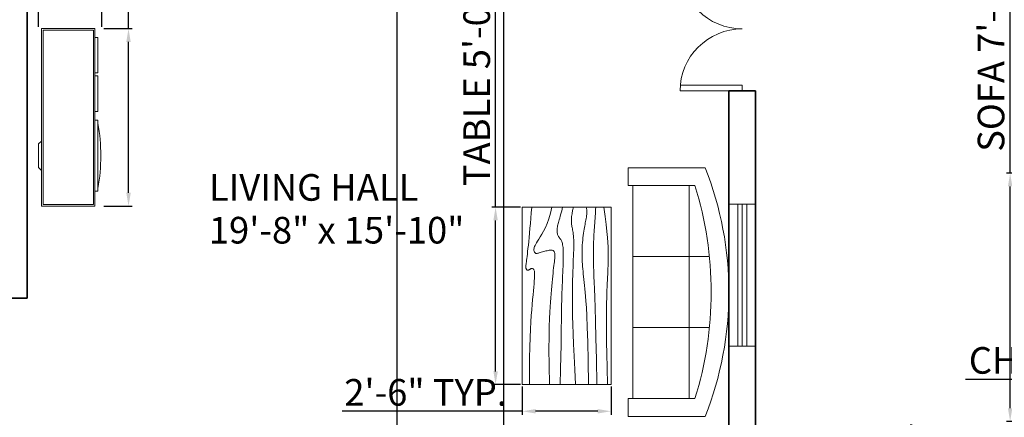
# Model space of a CAD drawing. Units: inches. Extents: x 2081 to 4786, y 1256 to 3802.
# Tile 4 of 7: x 2352 to 2685, y 1670 to 1804. Entities that reach past the tile are written whole.
import ezdxf

# ---------------------------------------------------------------- set-up
doc = ezdxf.new("R2010")
doc.units = ezdxf.units.IN
for name, color, linetype, lineweight in [('A-ANNO-DIMS', 18, 'Continuous', 18), ('A-AREA-IDEN', 18, 'Continuous', 18), ('A-DOOR', 5, 'Continuous', 18), ('A-FURN', 5, 'Continuous', 18), ('A-GLAZ', 11, 'Continuous', 18), ('A-WALL', 7, 'Continuous', 35)]:
    doc.layers.add(name, color=color, linetype=linetype, lineweight=lineweight)
doc.styles.get("Standard").update_dxf_attribs({"font": 'arial.ttf'})
doc.dimstyles.new('ISO-25', dxfattribs={"dimtxt": 9, "dimasz": 4.5, "dimexe": 1.25, "dimexo": 0.625, "dimtad": 1, "dimdec": 0, "dimlunit": 3, "dimtxsty": 'Standard', "dimcen": 2.5, "dimadec": 0, "dimazin": 0, "dimtfac": 1, "dimtdec": 0, "dimtmove": 0, "dimatfit": 3, "dimfxl": 1, "dimarcsym": 0})

# ---------------------------------------------------------------- blocks, each defined once
blk = doc.blocks.new('Sofa - Roundback 7 ft.')
for p, q in [((-12.00002, -32.4421), (-12.00003, -6.5971)), ((11.99997, -32.4421), (11.99998, -6.5971)), ((-36.000027, -34), (-36.000027, -11.4696)), ((35.99998, -34), (35.99998, -11.4696)), ((-35.999844, -13.3819), (35.9998, -13.3819)), ((-36.000027, -32.4421), (35.99998, -32.4421))]:
    blk.add_line(p, q)
for points in [[(-36.000027, -34), (-42.000027, -34), (-42.000027, -8)], [(41.99998, -8), (41.99998, -34), (35.99998, -34)]]:
    blk.add_lwpolyline(points)
for centre, radius, start, end in [((0, -114.25), 114.25, 68.43141, 111.5686), ((-0.00001, -127.1968), 121.1968, 72.72033, 107.2797)]:
    blk.add_arc(centre, radius, start, end)
blk = doc.blocks.new('Table - Rectangular Woodgrain 60 x 30 in.')
for p, q in [((0, 0), (0, -30)), ((60, 0), (0, 0)), ((60, -30), (60, 0)), ((0, -30), (60, -30))]:
    blk.add_line(p, q)
for points in [[(0, -2.4), (4.8155, -2.418), (9.0302, -2.4688), (12.709, -2.5477), (15.9167, -2.65), (18.7181, -2.7711), (21.1781, -2.9063), (23.3616, -3.0508), (25.3333, -3.2), (27.1477, -3.3495), (28.8172, -3.4958), (30.3437, -3.636), (31.7291, -3.7667), (32.9756, -3.8849), (34.0849, -3.9875), (35.059, -4.0714), (35.9, -4.1334), (36.6114, -4.1711), (37.2041, -4.1854), (37.6906, -4.1779), (38.0833, -4.15), (38.3948, -4.1034), (38.6375, -4.0396), (38.8239, -3.9602), (38.9666, -3.8667), (39.0764, -3.7608), (39.1573, -3.6448), (39.2116, -3.521), (39.2416, -3.3917), (39.2498, -3.2593), (39.2385, -3.1261), (39.21, -2.9944), (39.1666, -2.8667), (39.111, -2.7447), (39.0468, -2.6281), (38.978, -2.5163), (38.9083, -2.4083), (38.8418, -2.3035), (38.7823, -2.201), (38.7337, -2.1001), (38.7, -2), (38.6844, -1.9003), (38.6875, -1.8021), (38.7094, -1.707), (38.75, -1.6167), (38.8094, -1.5326), (38.8875, -1.4563), (38.9844, -1.3893), (39.1, -1.3333), (39.2351, -1.2896), (39.3937, -1.2583), (39.5804, -1.2396), (39.8, -1.2333), (40.057, -1.2396), (40.3562, -1.2583), (40.7023, -1.2896), (41.1, -1.3333), (41.5547, -1.3895), (42.0755, -1.4573), (42.6721, -1.5361), (43.3542, -1.625), (44.1316, -1.7233), (45.014, -1.8302), (46.0114, -1.9449), (47.1333, -2.0667), (48.3862, -2.1947), (49.7625, -2.3281), (51.2513, -2.4663), (52.8416, -2.6083), (54.5226, -2.7535), (56.2833, -2.9011), (58.1127, -3.0501), (60, -3.2)], [(0, -9.2), (6.5759, -9.0858), (11.9385, -9.0365), (16.2527, -9.0418), (19.6833, -9.0917), (22.3952, -9.1759), (24.5531, -9.2844), (26.322, -9.4069), (27.8666, -9.5333), (29.3241, -9.6553), (30.7203, -9.7719), (32.0532, -9.8837), (33.3208, -9.9917), (34.5213, -10.0965), (35.6526, -10.199), (36.7128, -10.2999), (37.7, -10.4), (38.6129, -10.4996), (39.4531, -10.5969), (40.223, -10.6895), (40.925, -10.775), (41.5613, -10.8512), (42.1344, -10.9156), (42.6465, -10.966), (43.1, -11), (43.4976, -11.0158), (43.8437, -11.0136), (44.143, -10.9942), (44.4, -10.9583), (44.6195, -10.9069), (44.8062, -10.8406), (44.9648, -10.7603), (45.1, -10.6667), (45.2155, -10.5598), (45.3114, -10.4365), (45.3871, -10.2929), (45.4416, -10.125), (45.4743, -9.929), (45.4844, -9.7011), (45.4709, -9.4371), (45.4333, -9.1333), (45.3716, -8.7883), (45.2896, -8.4104), (45.1919, -8.0107), (45.0833, -7.6), (44.9685, -7.1893), (44.8521, -6.7896), (44.7388, -6.4117), (44.6333, -6.0667), (44.54, -5.7628), (44.4614, -5.4979), (44.4001, -5.2675), (44.3583, -5.0667), (44.3384, -4.8909), (44.3427, -4.7354), (44.3736, -4.5956), (44.4333, -4.4667), (44.5236, -4.3453), (44.6427, -4.2333), (44.7884, -4.1339), (44.9583, -4.05), (45.1501, -3.9849), (45.3614, -3.9417), (45.59, -3.9234), (45.8333, -3.9333), (46.0915, -3.9749), (46.3734, -4.0531), (46.6906, -4.1736), (47.0542, -4.3417), (47.4756, -4.5629), (47.9661, -4.8427), (48.5372, -5.1866), (49.2, -5.6), (49.9676, -6.0844), (50.8594, -6.625), (51.8965, -7.2031), (53.1, -7.8), (54.491, -8.3969), (56.0906, -8.975), (57.9199, -9.5156), (60, -10)], [(0, -12.8), (5.1847, -12.9322), (9.6213, -13.0323), (13.3963, -13.1059), (16.5958, -13.1583), (19.3063, -13.1952), (21.614, -13.2219), (23.6054, -13.2439), (25.3666, -13.2667), (26.9728, -13.2947), (28.4531, -13.3281), (29.8256, -13.3663), (31.1083, -13.4083), (32.3191, -13.4535), (33.476, -13.501), (34.597, -13.5501), (35.7, -13.6), (36.7984, -13.6497), (37.8875, -13.6979), (38.9578, -13.743), (40, -13.7833), (41.0047, -13.8174), (41.9625, -13.8438), (42.864, -13.8607), (43.7, -13.8667), (44.4631, -13.8604), (45.1552, -13.8417), (45.7801, -13.8104), (46.3416, -13.7667), (46.8439, -13.7104), (47.2906, -13.6417), (47.6858, -13.5604), (48.0333, -13.4667), (48.3375, -13.3608), (48.6042, -13.2448), (48.8396, -13.121), (49.05, -12.9917), (49.2417, -12.8593), (49.4208, -12.7261), (49.5937, -12.5944), (49.7667, -12.4667), (49.9452, -12.3451), (50.1323, -12.2313), (50.3303, -12.1268), (50.5416, -12.0333), (50.7686, -11.9524), (51.0135, -11.8854), (51.2788, -11.8341), (51.5666, -11.8), (51.8785, -11.7843), (52.2116, -11.7865), (52.562, -11.8059), (52.926, -11.8417), (53.2998, -11.8931), (53.6795, -11.9594), (54.0614, -12.0397), (54.4416, -12.1333), (54.8223, -12.2401), (55.2293, -12.3625), (55.6942, -12.5037), (56.2489, -12.6667), (56.9251, -12.8547), (57.7545, -13.0708), (58.7689, -13.3182), (60, -13.6)], [(0, -18), (5.124, -17.7273), (9.6609, -17.5057), (13.6705, -17.3303), (17.2125, -17.1958), (20.3467, -17.0973), (23.1328, -17.0297), (25.6307, -16.9878), (27.9, -16.9667), (29.9928, -16.9617), (31.9302, -16.9703), (33.7254, -16.9907), (35.3917, -17.0208), (36.9423, -17.0588), (38.3906, -17.1026), (39.7499, -17.1503), (41.0333, -17.2), (42.2519, -17.2496), (43.4073, -17.2969), (44.4986, -17.3395), (45.525, -17.375), (46.4858, -17.4012), (47.3802, -17.4156), (48.2074, -17.416), (48.9667, -17.4), (49.6583, -17.3662), (50.2872, -17.3167), (50.8595, -17.2547), (51.3812, -17.1833), (51.8584, -17.1057), (52.2971, -17.025), (52.7034, -16.9443), (53.0833, -16.8667), (53.443, -16.7951), (53.789, -16.7313), (54.128, -16.6768), (54.4666, -16.6334), (54.8115, -16.6024), (55.1693, -16.5854), (55.5465, -16.5841), (55.95, -16.6), (56.3828, -16.6337), (56.8346, -16.6823), (57.2915, -16.7418), (57.7396, -16.8084), (58.165, -16.878), (58.5539, -16.9469), (58.8924, -17.0111), (59.1666, -17.0667), (59.3679, -17.1107), (59.5078, -17.1438), (59.6032, -17.1675), (59.6708, -17.1833), (59.7275, -17.193), (59.7901, -17.1979), (59.8753, -17.1998), (60, -17.2)], [(0, -22.4), (8.0098, -22.2501), (14.4094, -22.1011), (19.4168, -21.9535), (23.25, -21.8083), (26.1269, -21.6663), (28.2656, -21.5281), (29.884, -21.3947), (31.2, -21.2667), (32.3967, -21.1448), (33.5172, -21.0292), (34.5697, -20.9198), (35.5625, -20.8167), (36.5037, -20.7198), (37.4015, -20.6292), (38.2642, -20.5448), (39.1, -20.4667), (39.9164, -20.3951), (40.7187, -20.3313), (41.5117, -20.2768), (42.3, -20.2333), (43.0883, -20.2024), (43.8812, -20.1854), (44.6836, -20.1841), (45.5, -20.2), (46.3328, -20.234), (47.1747, -20.2844), (48.0163, -20.3488), (48.8479, -20.425), (49.66, -20.5106), (50.4429, -20.6031), (51.1872, -20.7004), (51.8833, -20.8), (52.5246, -20.8999), (53.1166, -20.9995), (53.6681, -21.0983), (54.1875, -21.1958), (54.6834, -21.2919), (55.1646, -21.3859), (55.6394, -21.4777), (56.1167, -21.5667), (56.6028, -21.6515), (57.0961, -21.7266), (57.5929, -21.7852), (58.0896, -21.8208), (58.5823, -21.8268), (59.0674, -21.7964), (59.5412, -21.723), (60, -21.6)], [(0, -25.2), (8.6355, -25.0504), (15.7026, -24.9031), (21.4049, -24.7606), (25.9458, -24.625), (29.529, -24.4988), (32.3578, -24.3844), (34.6359, -24.284), (36.5667, -24.2), (38.3213, -24.1341), (39.9417, -24.0854), (41.437, -24.0523), (42.8167, -24.0333), (44.0901, -24.0268), (45.2667, -24.0313), (46.3557, -24.0451), (47.3667, -24.0667), (48.309, -24.0947), (49.1928, -24.1287), (50.0284, -24.168), (50.826, -24.2125), (51.5959, -24.2617), (52.3483, -24.3151), (53.0935, -24.3725), (53.8417, -24.4334), (54.6009, -24.497), (55.3699, -24.561), (56.1454, -24.6226), (56.9239, -24.6792), (57.7021, -24.7279), (58.4764, -24.7662), (59.2435, -24.7911), (60, -24.8)], [(0, -28.8), (5.6867, -28.6681), (10.45, -28.5698), (14.407, -28.5012), (17.675, -28.4584), (20.3711, -28.4374), (22.6125, -28.4344), (24.5164, -28.4455), (26.2, -28.4667), (27.762, -28.4947), (29.2276, -28.5281), (30.6033, -28.5663), (31.8958, -28.6084), (33.1118, -28.6535), (34.2578, -28.7011), (35.3405, -28.7501), (36.3666, -28.8), (37.3443, -28.8497), (38.288, -28.8974), (39.2137, -28.9412), (40.1375, -28.9792), (41.0753, -29.0093), (42.0432, -29.0297), (43.0572, -29.0384), (44.1333, -29.0333), (45.2936, -29.0114), (46.5843, -28.9641), (48.0579, -28.8816), (49.7666, -28.7542), (51.7629, -28.5721), (54.0989, -28.3255), (56.8272, -28.0048), (60, -27.6)]]:
    blk.add_lwpolyline(points)
blk = doc.blocks.new('Entertainment Center')
for p, q in [((-4, 0), (-5, -1)), ((4, 0), (-4, 0)), ((5, -1), (4, 0)), ((-17, -19), (-17, -1)), ((-17, -1), (43, -1)), ((-16.5, -18.5), (-16.5, -1.5)), ((-16.5, -1.5), (42.5, -1.5)), ((42.5, -1.5), (42.5, -18.5)), ((43, -1), (43, -19)), ((43, -19), (-17, -19)), ((42.5, -18.5), (-16.5, -18.5)), ((-12, -20), (-12, -19)), ((12, -19), (12, -20)), ((15, -20), (15, -19)), ((27, -19), (27, -20)), ((28, -20), (28, -19)), ((40, -19), (40, -20)), ((12, -20), (-12, -20)), ((27, -20), (15, -20)), ((40, -20), (28, -20))]:
    blk.add_line(p, q)
blk.add_arc((0, 40), 61, 259.6111, 280.3889)
blk = doc.blocks.new('DOOR-PAIR-42IN')
for p, q in [((0, 42), (21, 42)), ((0, 40), (21, 40)), ((21, 42), (21, 40)), ((0, 2), (21, 2)), ((21, 0), (21, 2)), ((0, 0), (21, 0))]:
    blk.add_line(p, q)
for centre, start, end in [((21, 42), 180, 270), ((21, 0), 90, 180)]:
    blk.add_arc(centre, 21, start, end)
blk = doc.blocks.new('WINDOW-48IN')
for p, q in [((0, 0), (0, 9)), ((0, 9), (4, 9)), ((4, 9), (48, 9)), ((48, 0), (48, 9)), ((48, 6), (0, 6)), ((48, 4.5), (0, 4.5)), ((48, 3), (0, 3)), ((48, 0), (0, 0))]:
    blk.add_line(p, q)
blk = doc.blocks.new('*D51')
at = {"layer": 'A-ANNO-DIMS', "color": 0, "lineweight": -2, "transparency": 16777216}
for p, q in [((2744.09, 1682.64), (2671.91, 1682.64)), ((2744.09, 1677.68), (2744.09, 1683.89)), ((2776.84, 1682.64), (2748.59, 1682.64)), ((2781.34, 1677.68), (2781.34, 1683.89))]:
    blk.add_line(p, q, dxfattribs=at)
at = {"layer": 'A-ANNO-DIMS', "color": 0, "transparency": 16777216}
for points in [[(2748.59, 1683.39), (2748.59, 1681.89), (2744.09, 1682.64)], [(2776.84, 1683.39), (2776.84, 1681.89), (2781.34, 1682.64)]]:
    blk.add_solid(points, dxfattribs=at)
at = {"layer": 'Defpoints', "color": 0, "transparency": 16777216}
for p in [(2744.09, 1682.64), (2744.09, 1677.06), (2781.34, 1677.06)]:
    blk.add_point(p, dxfattribs=at)
at = {"layer": 'A-ANNO-DIMS', "color": 0, "transparency": 16777216, "insert": (2705.75, 1687.93), "char_height": 9, "attachment_point": 5}
blk.add_mtext('CHAIR 3\'-1"', dxfattribs=at)
blk = doc.blocks.new('*D55')
at = {"layer": 'A-ANNO-DIMS', "color": 0, "lineweight": -2, "transparency": 16777216}
for p, q in [((2686.95, 1752.41), (2686.95, 1850.7)), ((2698.93, 1752.41), (2685.7, 1752.41)), ((2686.95, 1672.91), (2686.95, 1747.91)), ((2698.93, 1668.41), (2685.7, 1668.41))]:
    blk.add_line(p, q, dxfattribs=at)
at = {"layer": 'A-ANNO-DIMS', "color": 0, "transparency": 16777216}
for points in [[(2686.2, 1747.91), (2687.7, 1747.91), (2686.95, 1752.41)], [(2686.2, 1672.91), (2687.7, 1672.91), (2686.95, 1668.41)]]:
    blk.add_solid(points, dxfattribs=at)
at = {"layer": 'Defpoints', "color": 0, "transparency": 16777216}
for p in [(2686.95, 1752.41), (2699.55, 1752.41), (2699.55, 1668.41)]:
    blk.add_point(p, dxfattribs=at)
at = {"layer": 'A-ANNO-DIMS', "color": 0, "transparency": 16777216, "insert": (2681.67, 1803.8), "char_height": 9, "attachment_point": 5, "rotation": 90}
blk.add_mtext('SOFA 7\'-0" TYP.', dxfattribs=at)
blk = doc.blocks.new('*D56')
at = {"layer": 'A-ANNO-DIMS', "color": 0, "lineweight": -2, "transparency": 16777216}
for p, q in [((2699.55, 1667.78), (2699.55, 1654.56)), ((2736.22, 1667.78), (2736.22, 1654.56)), ((2699.55, 1655.81), (2617.98, 1655.81)), ((2731.72, 1655.81), (2704.05, 1655.81))]:
    blk.add_line(p, q, dxfattribs=at)
at = {"layer": 'A-ANNO-DIMS', "color": 0, "transparency": 16777216}
for points in [[(2704.05, 1656.56), (2704.05, 1655.06), (2699.55, 1655.81)], [(2731.72, 1656.56), (2731.72, 1655.06), (2736.22, 1655.81)]]:
    blk.add_solid(points, dxfattribs=at)
at = {"layer": 'Defpoints', "color": 0, "transparency": 16777216}
for p in [(2699.55, 1668.41), (2736.22, 1668.41), (2699.55, 1655.81)]:
    blk.add_point(p, dxfattribs=at)
at = {"layer": 'A-ANNO-DIMS', "color": 0, "transparency": 16777216, "insert": (2656.52, 1661.09), "char_height": 9, "attachment_point": 5}
blk.add_mtext('3\'-0 1/2" TYP.', dxfattribs=at)
blk = doc.blocks.new('*D57')
at = {"layer": 'A-ANNO-DIMS', "color": 0, "lineweight": -2, "transparency": 16777216}
for p, q in [((2513.19, 1740.9), (2513.19, 1845.06)), ((2521.57, 1740.9), (2511.94, 1740.9)), ((2513.19, 1685.4), (2513.19, 1736.4)), ((2521.57, 1680.9), (2511.94, 1680.9))]:
    blk.add_line(p, q, dxfattribs=at)
at = {"layer": 'A-ANNO-DIMS', "color": 0, "transparency": 16777216}
for points in [[(2512.44, 1736.4), (2513.94, 1736.4), (2513.19, 1740.9)], [(2512.44, 1685.4), (2513.94, 1685.4), (2513.19, 1680.9)]]:
    blk.add_solid(points, dxfattribs=at)
at = {"layer": 'Defpoints', "color": 0, "transparency": 16777216}
for p in [(2513.19, 1740.9), (2522.19, 1740.9), (2522.19, 1680.9)]:
    blk.add_point(p, dxfattribs=at)
at = {"layer": 'A-ANNO-DIMS', "color": 0, "transparency": 16777216, "insert": (2507.97, 1795.23), "char_height": 9, "attachment_point": 5, "rotation": 90}
blk.add_mtext('TABLE 5\'-0" TYP.', dxfattribs=at)
blk = doc.blocks.new('*D58')
at = {"layer": 'A-ANNO-DIMS', "color": 0, "lineweight": -2, "transparency": 16777216}
for p, q in [((2522.19, 1680.27), (2522.19, 1670.65)), ((2552.19, 1680.27), (2552.19, 1670.65)), ((2522.19, 1671.9), (2461.43, 1671.9)), ((2547.69, 1671.9), (2526.69, 1671.9))]:
    blk.add_line(p, q, dxfattribs=at)
at = {"layer": 'A-ANNO-DIMS', "color": 0, "transparency": 16777216}
for points in [[(2526.69, 1672.65), (2526.69, 1671.15), (2522.19, 1671.9)], [(2547.69, 1672.65), (2547.69, 1671.15), (2552.19, 1671.9)]]:
    blk.add_solid(points, dxfattribs=at)
at = {"layer": 'Defpoints', "color": 0, "transparency": 16777216}
for p in [(2522.19, 1680.9), (2552.19, 1680.9), (2522.19, 1671.9)]:
    blk.add_point(p, dxfattribs=at)
at = {"layer": 'A-ANNO-DIMS', "color": 0, "transparency": 16777216, "insert": (2489.56, 1677.12), "char_height": 9, "attachment_point": 5}
blk.add_mtext('2\'-6" TYP.', dxfattribs=at)
blk = doc.blocks.new('*D59')
at = {"layer": 'A-ANNO-DIMS', "color": 0, "lineweight": -2, "transparency": 16777216}
for p, q in [((2389.23, 1801.25), (2389.23, 1937.59)), ((2380.85, 1801.25), (2390.48, 1801.25)), ((2389.23, 1745.75), (2389.23, 1796.75)), ((2380.85, 1741.25), (2390.48, 1741.25))]:
    blk.add_line(p, q, dxfattribs=at)
at = {"layer": 'A-ANNO-DIMS', "color": 0, "transparency": 16777216}
for points in [[(2388.48, 1796.75), (2389.98, 1796.75), (2389.23, 1801.25)], [(2388.48, 1745.75), (2389.98, 1745.75), (2389.23, 1741.25)]]:
    blk.add_solid(points, dxfattribs=at)
at = {"layer": 'Defpoints', "color": 0, "transparency": 16777216}
for p in [(2380.23, 1801.25), (2389.23, 1801.25), (2380.23, 1741.25)]:
    blk.add_point(p, dxfattribs=at)
at = {"layer": 'A-ANNO-DIMS', "color": 0, "transparency": 16777216, "insert": (2384.01, 1871.67), "char_height": 9, "attachment_point": 5, "rotation": 90}
blk.add_mtext('MEDIA UNIT 5\'-0" TYP.', dxfattribs=at)
blk = doc.blocks.new('*D60')
at = {"layer": 'A-ANNO-DIMS', "color": 0, "lineweight": -2, "transparency": 16777216}
for p, q in [((2358.89, 1810.25), (2278.16, 1810.25)), ((2358.89, 1801.88), (2358.89, 1811.5)), ((2375.73, 1810.25), (2363.39, 1810.25)), ((2380.23, 1801.88), (2380.23, 1811.5))]:
    blk.add_line(p, q, dxfattribs=at)
at = {"layer": 'A-ANNO-DIMS', "color": 0, "transparency": 16777216}
for points in [[(2363.39, 1811), (2363.39, 1809.5), (2358.89, 1810.25)], [(2375.73, 1811), (2375.73, 1809.5), (2380.23, 1810.25)]]:
    blk.add_solid(points, dxfattribs=at)
at = {"layer": 'Defpoints', "color": 0, "transparency": 16777216}
for p in [(2358.89, 1810.25), (2358.89, 1801.25), (2380.23, 1801.25)]:
    blk.add_point(p, dxfattribs=at)
at = {"layer": 'A-ANNO-DIMS', "color": 0, "transparency": 16777216, "insert": (2316.28, 1815.53), "char_height": 9, "attachment_point": 5}
blk.add_mtext('1\'-9 1/2" TYP.', dxfattribs=at)
blk = doc.blocks.new('*D78')
at = {"layer": 'A-ANNO-DIMS', "color": 0, "lineweight": -2, "transparency": 16777216}
for p, q in [((2479.98, 1626.8), (2479.98, 2072.92)), ((2484.48, 2071.67), (2511.48, 2071.67)), ((2515.98, 1639.8), (2515.98, 2072.92))]:
    blk.add_line(p, q, dxfattribs=at)
at = {"layer": 'A-ANNO-DIMS', "color": 0, "transparency": 16777216}
for points in [[(2484.48, 2072.42), (2484.48, 2070.92), (2479.98, 2071.67)], [(2511.48, 2072.42), (2511.48, 2070.92), (2515.98, 2071.67)]]:
    blk.add_solid(points, dxfattribs=at)
at = {"layer": 'Defpoints', "color": 0, "transparency": 16777216}
for p in [(2515.98, 2071.67), (2515.98, 1639.17), (2479.98, 1626.17)]:
    blk.add_point(p, dxfattribs=at)
at = {"layer": 'A-ANNO-DIMS', "color": 0, "transparency": 16777216, "insert": (2497.98, 2076.9), "char_height": 9, "attachment_point": 5}
blk.add_mtext('3\'-0"', dxfattribs=at)

msp = doc.modelspace()

# ---------------------------------------------------------------- linework, layer by layer
at = {"layer": 'A-WALL'}
for p, q in [((2354.98, 1710.17), (2354.98, 1834.17)), ((2591.98, 1780.17), (2600.98, 1780.17)), ((2591.98, 1644.17), (2591.98, 1780.17)), ((2600.98, 1433.17), (2600.98, 1780.17)), ((2343.98, 1710.17), (2354.98, 1710.17))]:
    msp.add_line(p, q, dxfattribs=at)

# ---------------------------------------------------------------- block references
at = {"layer": 'A-DOOR'}
msp.add_blockref('DOOR-PAIR-42IN', (2575.48, 1780.17), dxfattribs=at)
at = {"layer": 'A-FURN'}
for name, p, rotation in [('Entertainment Center', (2358.89, 1758.25), 90), ('Sofa - Roundback 7 ft.', (2591.98, 1712.17), 270), ('Table - Rectangular Woodgrain 60 x 30 in.', (2522.19, 1680.9), 90)]:
    msp.add_blockref(name, p, dxfattribs=dict(at, rotation=rotation))
at = {"layer": 'A-GLAZ', "rotation": 269.9999999999987}
msp.add_blockref('WINDOW-48IN', (2591.98, 1741.91), dxfattribs=at)

# ---------------------------------------------------------------- texts
at = {"layer": 'A-AREA-IDEN'}
for s, p in [('LIVING HALL', (2416.37, 1743.07)), ('19\'-8" x 15\'-10"', (2416.37, 1728.61))]:
    msp.add_text(s, height=9, dxfattribs=at).set_placement(p)

# ---------------------------------------------------------------- dimensions: what is measured, and where the dimension line sits
at = {"layer": 'A-ANNO-DIMS'}
dim = msp.add_linear_dim(base=(2515.98, 2071.67), p1=(2479.98, 1626.17), p2=(2515.98, 1639.17), dimstyle='ISO-25', override={"dimdec": 1, "dimlfac": 1, "dimrnd": 0, "dimzin": 1, "dimdsep": 46, "dimlunit": 4, "dimfrac": 2}, dxfattribs=at)
dim.commit()
dim.dimension.update_dxf_attribs({"geometry": '*D78', "text_midpoint": (2497.98, 2076.9)})
for base, p1, p2, angle, text, picture, middle in [((2389.23, 1801.25), (2380.23, 1741.25), (2380.23, 1801.25), 90, 'MEDIA UNIT <> TYP.', '*D59', (2384.01, 1871.67)), ((2686.95, 1752.41), (2699.55, 1668.41), (2699.55, 1752.41), 90, 'SOFA <> TYP.', '*D55', (2681.67, 1803.8)), ((2513.19, 1740.9), (2522.19, 1680.9), (2522.19, 1740.9), 90, 'TABLE <> TYP.', '*D57', (2507.97, 1795.23)), ((2358.89, 1810.25), (2380.23, 1801.25), (2358.89, 1801.25), 180, '<> TYP.', '*D60', (2316.28, 1815.53)), ((2744.0897, 1682.6449), (2781.3368, 1677.0579), (2744.0897, 1677.0579), 180, 'CHAIR <>', '*D51', (2705.7488, 1687.9265)), ((2522.19, 1671.9), (2552.19, 1680.9), (2522.19, 1680.9), 180, '<> TYP.', '*D58', (2489.56, 1677.12)), ((2699.55, 1655.81), (2736.22, 1668.41), (2699.55, 1668.41), 180, '<> TYP.', '*D56', (2656.52, 1661.09))]:
    dim = msp.add_linear_dim(base=base, p1=p1, p2=p2, angle=angle, text=text, dimstyle='ISO-25', override={"dimdec": 1, "dimlfac": 1, "dimrnd": 0, "dimzin": 1, "dimdsep": 46, "dimlunit": 4, "dimfrac": 2}, dxfattribs=at)
    dim.commit()
    dim.dimension.update_dxf_attribs({"geometry": picture, "text_midpoint": middle})

doc.saveas('drawing.dxf')
